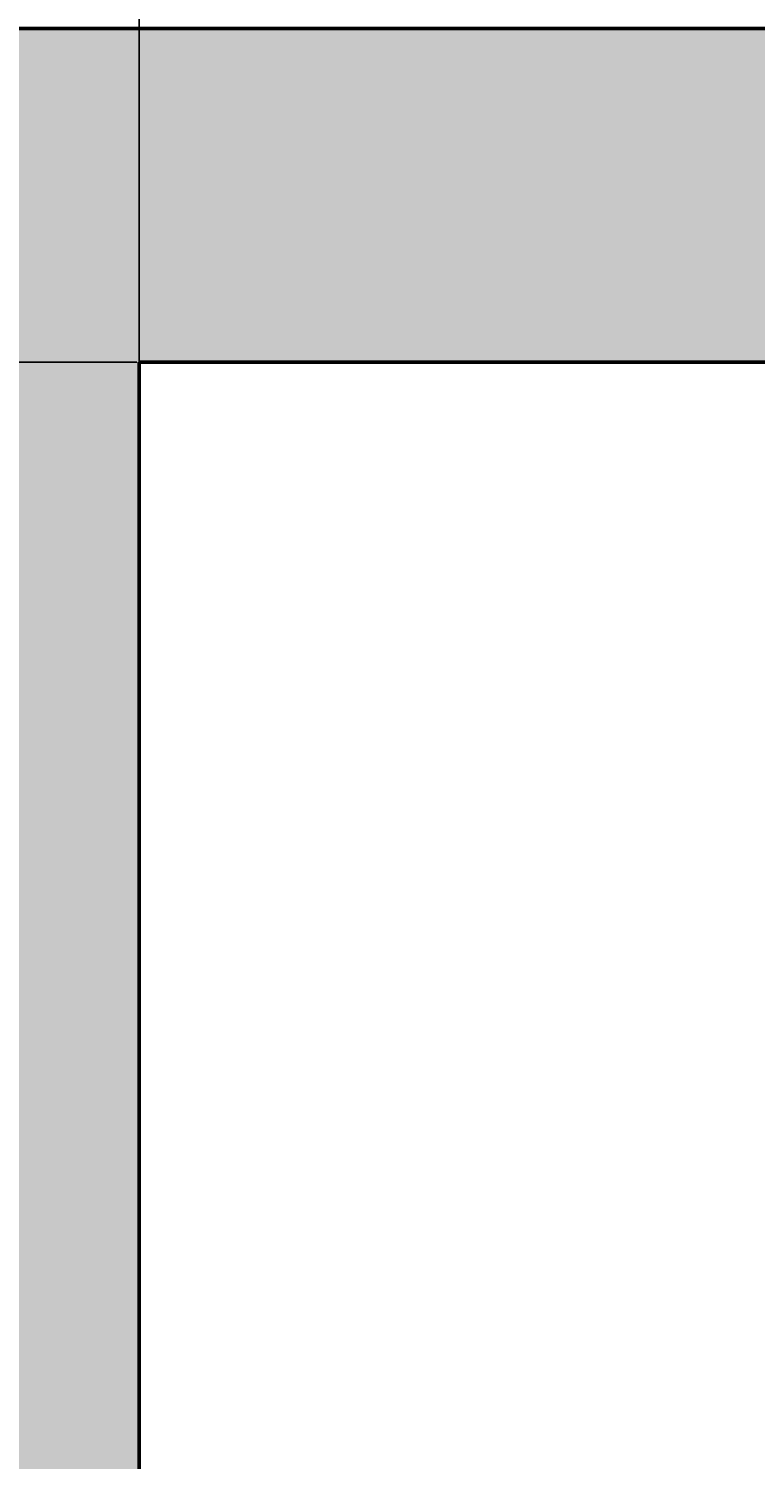
# Model space of a CAD drawing. Units: inches. Extents: x 2307 to 2544, y 2171 to 2540.
# Tile 45 of 52: x 2453 to 2472, y 2482 to 2521. Entities that reach past the tile are written whole.
import ezdxf

# ---------------------------------------------------------------- set-up
doc = ezdxf.new("R2010")
doc.units = ezdxf.units.IN
doc.layers.add('A-ANNO-DIMS', color=2, linetype='Continuous', lineweight=18)
doc.layers.add('A-WALL', color=7, linetype='Continuous', lineweight=50)
doc.layers.add('A-WALL-PATT', color=18, linetype='Continuous', lineweight=13, true_color=0x000000)
doc.styles.get("Standard").update_dxf_attribs({"font": 'arial.ttf'})
doc.dimstyles.get("Standard").update_dxf_attribs({"dimtxt": 0.18, "dimasz": 0.18, "dimexe": 0.18, "dimexo": 0.0625, "dimgap": 0.09, "dimtad": 0, "dimtih": 1, "dimtoh": 1, "dimdec": 4, "dimzin": 0, "dimdsep": 46, "dimtxsty": 'Standard', "dimcen": 0.09, "dimadec": 0, "dimazin": 0, "dimtfac": 1, "dimtdec": 4, "dimtofl": 0, "dimtmove": 0, "dimatfit": 3, "dimfxl": 1, "dimtolj": 1, "dimtzin": 0, "dimarcsym": 0})

# ---------------------------------------------------------------- blocks, each defined once
blk = doc.blocks.new('*D46')
at = {"layer": 'A-ANNO-DIMS', "color": 0, "lineweight": -2, "transparency": 16777216}
for p, q in [((2455.696, 2511.572), (2455.696, 2540.345)), ((2455.876, 2540.165), (2485.477, 2540.165)), ((2515.516, 2540.165), (2485.915, 2540.165)), ((2515.696, 2511.572), (2515.696, 2540.345))]:
    blk.add_line(p, q, dxfattribs=at)
at = {"layer": 'A-ANNO-DIMS', "color": 0, "transparency": 16777216}
for points in [[(2455.876, 2540.195), (2455.876, 2540.135), (2455.696, 2540.165)], [(2515.516, 2540.195), (2515.516, 2540.135), (2515.696, 2540.165)]]:
    blk.add_solid(points, dxfattribs=at)
at = {"layer": 'Defpoints', "color": 0, "transparency": 16777216}
for p in [(2515.696, 2540.165), (2455.696, 2511.51), (2515.696, 2511.51)]:
    blk.add_point(p, dxfattribs=at)
at = {"layer": 'A-ANNO-DIMS', "color": 0, "transparency": 16777216, "insert": (2485.696, 2540.165), "char_height": 0.18, "attachment_point": 5}
blk.add_mtext('\\A1;60', dxfattribs=at)
blk = doc.blocks.new('*D48')
at = {"layer": 'A-ANNO-DIMS', "color": 0, "lineweight": -2, "transparency": 16777216}
for p, q in [((2455.633, 2511.51), (2307.366, 2511.51)), ((2307.546, 2511.33), (2307.546, 2475.69)), ((2307.546, 2439.69), (2307.546, 2475.329)), ((2455.633, 2439.51), (2307.366, 2439.51))]:
    blk.add_line(p, q, dxfattribs=at)
at = {"layer": 'A-ANNO-DIMS', "color": 0, "transparency": 16777216}
for points in [[(2307.516, 2511.33), (2307.576, 2511.33), (2307.546, 2511.51)], [(2307.516, 2439.69), (2307.576, 2439.69), (2307.546, 2439.51)]]:
    blk.add_solid(points, dxfattribs=at)
at = {"layer": 'Defpoints', "color": 0, "transparency": 16777216}
for p in [(2307.546, 2511.51), (2455.696, 2511.51), (2455.696, 2439.51)]:
    blk.add_point(p, dxfattribs=at)
at = {"layer": 'A-ANNO-DIMS', "color": 0, "transparency": 16777216, "insert": (2307.546, 2475.51), "char_height": 0.18, "attachment_point": 5}
blk.add_mtext('\\A1;72', dxfattribs=at)
blk = doc.blocks.new('*D59')
at = {"layer": 'A-ANNO-DIMS', "color": 0, "lineweight": -2, "transparency": 16777216}
for p, q in [((2455.696, 2315.572), (2455.696, 2540.345)), ((2455.876, 2540.165), (2470.477, 2540.165)), ((2485.516, 2540.165), (2470.914, 2540.165)), ((2485.696, 2315.572), (2485.696, 2540.345))]:
    blk.add_line(p, q, dxfattribs=at)
at = {"layer": 'A-ANNO-DIMS', "color": 0, "transparency": 16777216}
for points in [[(2455.876, 2540.195), (2455.876, 2540.135), (2455.696, 2540.165)], [(2485.516, 2540.195), (2485.516, 2540.135), (2485.696, 2540.165)]]:
    blk.add_solid(points, dxfattribs=at)
at = {"layer": 'Defpoints', "color": 0, "transparency": 16777216}
for p in [(2455.696, 2540.165), (2455.696, 2315.51), (2485.696, 2315.51)]:
    blk.add_point(p, dxfattribs=at)
at = {"layer": 'A-ANNO-DIMS', "color": 0, "transparency": 16777216, "insert": (2470.696, 2540.165), "char_height": 0.18, "attachment_point": 5}
blk.add_mtext('\\A1;30', dxfattribs=at)

msp = doc.modelspace()

# ---------------------------------------------------------------- hatches: boundary and pattern name
at = {"layer": 'A-WALL-PATT'}
h = msp.add_hatch(color=256, dxfattribs=at)
h.dxf.hatch_style = 1
h.paths.add_polyline_path([(2433.6935, 2199.5096), (2415.6423, 2199.5096), (2415.6423, 2190.5096), (2433.7832, 2190.5096)], flags=17)
h.paths.add_polyline_path([(2367.6423, 2199.5096), (2335.6958, 2199.5096), (2335.6958, 2307.3983), (2326.6958, 2307.3983), (2326.6958, 2190.5096), (2367.6423, 2190.5096)])
h.paths.add_polyline_path([(2524.6958, 2520.5096), (2496.7832, 2520.5096), (2496.7832, 2515.5149), (2472.7832, 2515.5149), (2472.7832, 2520.5096), (2415.4028, 2520.5096), (2415.4028, 2511.5096), (2451.6958, 2511.5096), (2451.6958, 2439.5096), (2451.6958, 2391.5096), (2445.6958, 2391.5096), (2445.6958, 2387.5096), (2455.6958, 2387.5096), (2455.6958, 2435.5096), (2461.6958, 2435.5096), (2461.6958, 2439.5096), (2455.6958, 2439.5096), (2455.6958, 2511.5096), (2515.6958, 2511.5096), (2515.6958, 2439.5096), (2491.6958, 2439.5096), (2491.6958, 2435.5096), (2515.6958, 2435.5096), (2515.6958, 2319.5096), (2451.6958, 2319.5096), (2451.6958, 2281.5096), (2481.6958, 2281.5096), (2481.6958, 2225.5096), (2485.6958, 2225.5096), (2485.6958, 2285.5096), (2455.6958, 2285.5096), (2455.6958, 2315.5096), (2515.6958, 2315.5096), (2515.6958, 2199.5096), (2469.6952, 2199.5096), (2469.785, 2190.5096), (2524.6958, 2190.5096)])

# ---------------------------------------------------------------- linework, layer by layer
at = {"layer": 'A-WALL'}
for p, q in [((2455.6958, 2511.5096), (2515.6958, 2511.5096)), ((2455.6958, 2439.5096), (2455.6958, 2511.5096))]:
    msp.add_line(p, q, dxfattribs=at)
msp.add_lwpolyline([(2433.7832, 2190.5096), (2326.6958, 2190.5096), (2326.6958, 2520.5096), (2524.6958, 2520.5096), (2524.6958, 2190.5096), (2469.785, 2190.5096)], dxfattribs=at)

# ---------------------------------------------------------------- dimensions: what is measured, and where the dimension line sits
at = {"layer": 'A-ANNO-DIMS'}
for base, p1, p2, picture, middle in [((2515.6958, 2540.1649), (2455.6958, 2511.5096), (2515.6958, 2511.5096), '*D46', (2485.6958, 2540.1649)), ((2455.6958, 2540.1649), (2485.6958, 2315.5096), (2455.6958, 2315.5096), '*D59', (2470.6958, 2540.1649))]:
    dim = msp.add_linear_dim(base=base, p1=p1, p2=p2, dimstyle='Standard', override={"dimdec": 0, "dimlfac": 1, "dimrnd": 0, "dimzin": 0, "dimdsep": 46, "dimlunit": 2}, dxfattribs=at)
    dim.commit()
    dim.dimension.update_dxf_attribs({"geometry": picture, "text_midpoint": middle})
dim = msp.add_linear_dim(base=(2307.5458, 2511.5096), p1=(2455.6958, 2439.5096), p2=(2455.6958, 2511.5096), angle=90, dimstyle='Standard', override={"dimdec": 0, "dimlfac": 1, "dimrnd": 0, "dimzin": 0, "dimdsep": 46, "dimlunit": 2}, dxfattribs=at)
dim.commit()
dim.dimension.update_dxf_attribs({"geometry": '*D48', "text_midpoint": (2307.5458, 2475.5096)})

doc.saveas('drawing.dxf')
